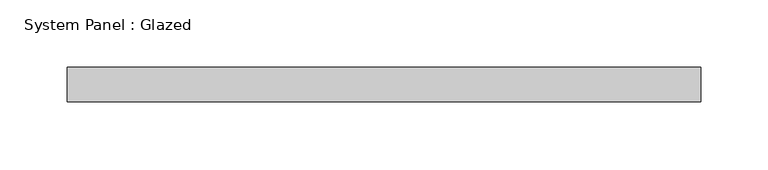
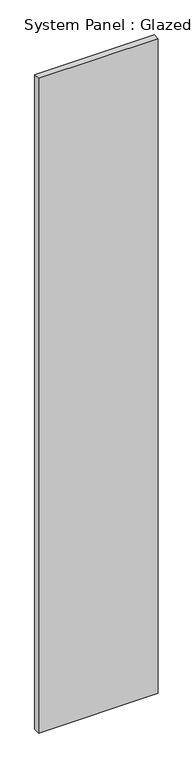
"""IFC4 building model written with IfcOpenShell, lengths in millimetres: plate geometry, System Panel : Glazed."""

from ifc_helpers import new_model, si_unit, origin, origin_with_axes, place, context, project, spatial, polyline, outline, extrude, source, transform, mapped, element, save


def system_panel_glazed_fd82e51e(model_context):
    return source(origin(), model_context, "Body", "SweptSolid", [
        extrude(outline(polyline([(234.95, 19.05), (-234.95, 19.05), (-234.95, 44.45), (234.95, 44.45), (234.95, 19.05)])), origin_with_axes(), (0.0, 0.0, 1.0), 2719.788773),
    ])


if __name__ == "__main__":
    model = new_model("IFC4")
    model_context = context("Model", 3, world=origin())
    ifc_project = project(units=[si_unit("LENGTHUNIT", "METRE", prefix="MILLI")], contexts=[model_context])
    site = spatial("IfcSite", under=ifc_project)
    building = spatial("IfcBuilding", under=site)
    placement = place(None, origin())
    system_panel_glazed_shape = system_panel_glazed_fd82e51e(model_context)
    element("IfcPlate", 1, ObjectType="System Panel : Glazed", at=placement, inside=building, context=model_context, shape_type="MappedRepresentation", body=[
        mapped(system_panel_glazed_shape, transform((0.0, 0.0, 0.0), x_axis=(1.0, 0.0, 0.0), y_axis=(0.0, 1.0, 0.0), z_axis=(0.0, 0.0, 1.0))),
    ])
    save(model, "model.ifc")

# Revit data of these elements
# Type "System Panel : Glazed"
#   Construction Type Id = "GSP4R"
#   Analytic Construction = "1/8 in Pilkington single glazing"
#   Visual Light Transmittance = 0.9
#   Solar Heat Gain Coefficient = 0.86
#   Heat Transfer Coefficient (U) = 1.18115 BTU/(h·ft²·°F)
# Element 1 (IfcPlate, "System Panel : Glazed")
#   Materials on its faces: "Glass"
# Materials
#   "Glass": class "Glass", colour RGB 0 128 192, transparency 0.75, Description = "Soda Lime Glass", Cost = 0
